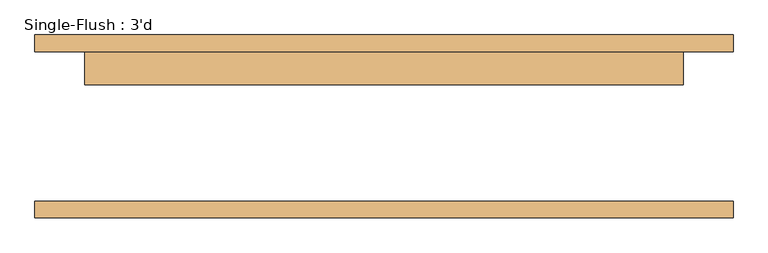
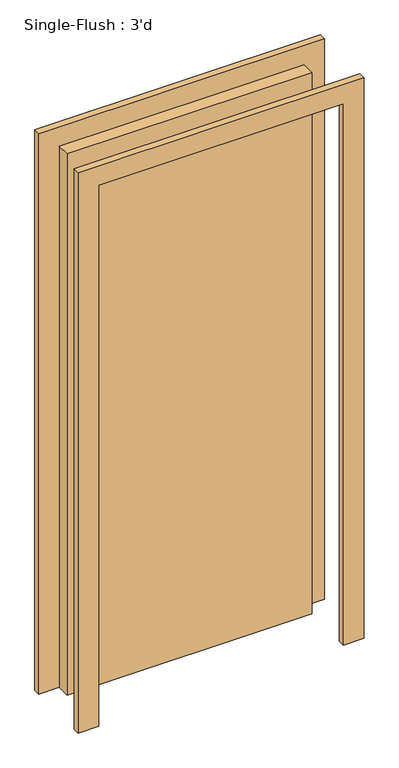
"""IFC4 building model written with IfcOpenShell, lengths in millimetres: door geometry, Single-Flush : 3'd."""

from ifc_helpers import new_model, si_unit, frame, origin, origin_with_axes, place, context, project, spatial, polyline, outline, extrude, source, transform, mapped, element, save


def single_flush_3_d_0ca8825f(model_context):
    return source(origin(), model_context, "Body", "SweptSolid", [
        extrude(outline(polyline([(2209.8, -533.4), (0.0, -533.4), (0.0, -457.2), (2133.6, -457.2), (2133.6, 457.2), (0.0, 457.2), (0.0, 533.4), (2209.8, 533.4), (2209.8, -533.4)])), frame((0.0, 114.3, 0.0), z_axis=(0.0, 1.0, 0.0), x_axis=(0.0, 0.0, 1.0)), (0.0, 0.0, 1.0), 25.4),
        extrude(outline(polyline([(2209.8, 533.4), (2209.8, -533.4), (0.0, -533.4), (0.0, -457.2), (2133.6, -457.2), (2133.6, 457.2), (0.0, 457.2), (0.0, 533.4), (2209.8, 533.4)])), frame((0.0, -139.7, 0.0), z_axis=(0.0, 1.0, 0.0), x_axis=(0.0, 0.0, 1.0)), (0.0, 0.0, 1.0), 25.4),
        extrude(outline(polyline([(457.2, 63.5), (-457.2, 63.5), (-457.2, 114.3), (457.2, 114.3), (457.2, 63.5)])), origin_with_axes(), (0.0, 0.0, 1.0), 2133.6),
    ])


if __name__ == "__main__":
    model = new_model("IFC4")
    model_context = context("Model", 3, world=origin())
    ifc_project = project(units=[si_unit("LENGTHUNIT", "METRE", prefix="MILLI")], contexts=[model_context])
    site = spatial("IfcSite", under=ifc_project)
    building = spatial("IfcBuilding", under=site)
    placement = place(None, origin())
    single_flush_3_d_shape = single_flush_3_d_0ca8825f(model_context)
    element("IfcDoor", 1, ObjectType="Single-Flush : 3'd", at=placement, inside=building, context=model_context, shape_type="MappedRepresentation", body=[
        mapped(single_flush_3_d_shape, transform((0.0, 0.0, 0.0), x_axis=(1.0, 0.0, 0.0), y_axis=(0.0, 1.0, 0.0), z_axis=(0.0, 0.0, 1.0))),
    ])
    save(model, "model.ifc")

# Revit data of these elements
# Type "Single-Flush : 3'd"
#   Type Mark = "13"
#   Construction Type Id = "MDOOR"
#   Assembly Code = "C1020"
#   Analytic Construction = "Metal"
#   Thickness = 0' - 2"
#   Heat Transfer Coefficient (U) = 0.651978 BTU/(h·ft²·°F)
#   Height = 7' - 0"
#   Trim Projection Ext = 0' - 1"
#   Trim Projection Int = 0' - 1"
#   Trim Width = 0' - 3"
#   Width = 3' - 0"
#   Define Thermal Properties by = 1
#   Door Material = Door - Panel
#   Frame Material = Door - Frame
#   Visual Light Transmittance = 0
#   Solar Heat Gain Coefficient = 0
#   Function = (empty or 0)
#   Wall Closure = (empty or 0)
# Element 1 (IfcDoor, "Single-Flush : 3'd")
#   Materials on its faces: "Door - Frame", "Door - Panel"
# Materials
#   "Door - Panel": class "Wood", colour RGB 210 159 95, transparency 0, Cost = 0
#   "Door - Frame": colour RGB 118 70 51, transparency 0, Cost = 0
